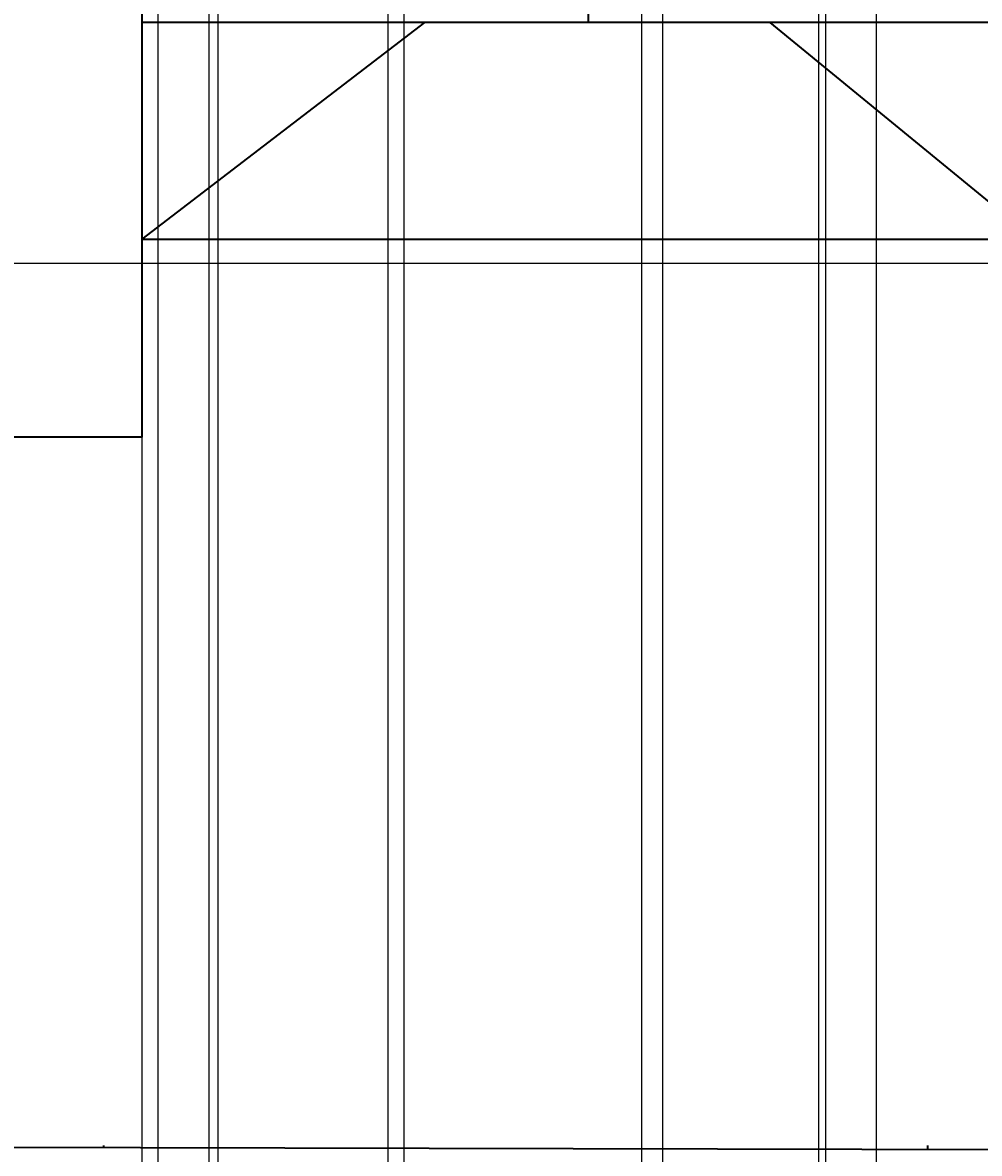
# Model space of a CAD drawing. Units: inches. Extents: x 27 to 200, y -50 to 102.
# Tile 17 of 26: x 117 to 145, y 19 to 52. Entities that reach past the tile are written whole.
import ezdxf

# ---------------------------------------------------------------- set-up
doc = ezdxf.new("R2010")
doc.units = ezdxf.units.IN
doc.header["$MEASUREMENT"] = 0
doc.layers.add('A-ANNO-DIMS', color=2, linetype='Continuous', lineweight=18)
doc.layers.add('A-ELEV', color=7, linetype='Continuous', lineweight=35)
doc.styles.get("Standard").update_dxf_attribs({"font": 'arial.ttf'})
doc.dimstyles.get("Standard").update_dxf_attribs({"dimtxt": 0.18, "dimasz": 0.18, "dimexe": 0.18, "dimexo": 0.0625, "dimgap": 0.09, "dimtad": 0, "dimtih": 1, "dimtoh": 1, "dimdec": 4, "dimzin": 0, "dimdsep": 46, "dimtxsty": 'Standard', "dimcen": 0.09, "dimadec": 0, "dimazin": 0, "dimtfac": 1, "dimtdec": 4, "dimtofl": 0, "dimtmove": 0, "dimatfit": 3, "dimfxl": 1, "dimtolj": 1, "dimtzin": 0, "dimarcsym": 0})

# ---------------------------------------------------------------- blocks, each defined once
blk = doc.blocks.new('*D48')
at = {"layer": 'A-ANNO-DIMS', "color": 0, "lineweight": -2, "transparency": 16777216}
for p, q in [((84.479, 44.926), (199.797, 44.926)), ((199.617, 44.746), (199.617, 14.26)), ((199.617, -16.589), (199.617, 13.897)), ((84.479, -16.769), (199.797, -16.769))]:
    blk.add_line(p, q, dxfattribs=at)
at = {"layer": 'A-ANNO-DIMS', "color": 0, "transparency": 16777216}
for points in [[(199.587, 44.746), (199.647, 44.746), (199.617, 44.926)], [(199.587, -16.589), (199.647, -16.589), (199.617, -16.769)]]:
    blk.add_solid(points, dxfattribs=at)
at = {"layer": 'Defpoints', "color": 0, "transparency": 16777216}
for p in [(84.417, 44.926), (199.617, 44.926), (84.417, -16.769)]:
    blk.add_point(p, dxfattribs=at)
at = {"layer": 'A-ANNO-DIMS', "color": 0, "transparency": 16777216, "insert": (199.617, 14.079), "char_height": 0.18, "attachment_point": 5}
blk.add_mtext('\\A1;61.7', dxfattribs=at)
blk = doc.blocks.new('*D51')
at = {"layer": 'A-ANNO-DIMS', "color": 0, "lineweight": -2, "transparency": 16777216}
for p, q in [((120.417, 45.561), (120.417, -25.149)), ((146.417, 45.561), (146.417, -25.149)), ((120.597, -24.969), (133.197, -24.969)), ((146.237, -24.969), (133.637, -24.969))]:
    blk.add_line(p, q, dxfattribs=at)
at = {"layer": 'A-ANNO-DIMS', "color": 0, "transparency": 16777216}
for points in [[(120.597, -24.939), (120.597, -24.999), (120.417, -24.969)], [(146.237, -24.939), (146.237, -24.999), (146.417, -24.969)]]:
    blk.add_solid(points, dxfattribs=at)
at = {"layer": 'Defpoints', "color": 0, "transparency": 16777216}
for p in [(120.417, 45.623), (146.417, 45.623), (146.417, -24.969)]:
    blk.add_point(p, dxfattribs=at)
at = {"layer": 'A-ANNO-DIMS', "color": 0, "transparency": 16777216, "insert": (133.417, -24.969), "char_height": 0.18, "attachment_point": 5}
blk.add_mtext('\\A1;26', dxfattribs=at)
blk = doc.blocks.new('*D53')
at = {"layer": 'A-ANNO-DIMS', "color": 0, "lineweight": -2, "transparency": 16777216}
for p, q in [((120.895, 14.04), (120.895, 102.306)), ((121.075, 102.126), (130.962, 102.126)), ((141.636, 102.126), (131.75, 102.126)), ((141.816, 14.04), (141.816, 102.306))]:
    blk.add_line(p, q, dxfattribs=at)
at = {"layer": 'A-ANNO-DIMS', "color": 0, "transparency": 16777216}
for points in [[(121.075, 102.156), (121.075, 102.096), (120.895, 102.126)], [(141.636, 102.156), (141.636, 102.096), (141.816, 102.126)]]:
    blk.add_solid(points, dxfattribs=at)
at = {"layer": 'Defpoints', "color": 0, "transparency": 16777216}
for p in [(141.816, 102.126), (120.895, 13.977), (141.816, 13.977)]:
    blk.add_point(p, dxfattribs=at)
at = {"layer": 'A-ANNO-DIMS', "color": 0, "transparency": 16777216, "insert": (131.356, 102.126), "char_height": 0.18, "attachment_point": 5}
blk.add_mtext('\\A1;20.92', dxfattribs=at)
blk = doc.blocks.new('*D57')
at = {"layer": 'A-ANNO-DIMS', "color": 0, "lineweight": -2, "transparency": 16777216}
for p, q in [((122.38, 4.48), (122.38, 102.306)), ((122.56, 102.126), (130.875, 102.126)), ((139.961, 102.126), (131.645, 102.126)), ((140.141, 4.48), (140.141, 102.306))]:
    blk.add_line(p, q, dxfattribs=at)
at = {"layer": 'A-ANNO-DIMS', "color": 0, "transparency": 16777216}
for points in [[(122.56, 102.156), (122.56, 102.096), (122.38, 102.126)], [(139.961, 102.156), (139.961, 102.096), (140.141, 102.126)]]:
    blk.add_solid(points, dxfattribs=at)
at = {"layer": 'Defpoints', "color": 0, "transparency": 16777216}
for p in [(140.141, 102.126), (122.38, 4.418), (140.141, 4.418)]:
    blk.add_point(p, dxfattribs=at)
at = {"layer": 'A-ANNO-DIMS', "color": 0, "transparency": 16777216, "insert": (131.26, 102.126), "char_height": 0.18, "attachment_point": 5}
blk.add_mtext('\\A1;17.76', dxfattribs=at)
blk = doc.blocks.new('*D59')
at = {"layer": 'A-ANNO-DIMS', "color": 0, "lineweight": -2, "transparency": 16777216}
for p, q in [((127.595, -0.162), (127.595, 102.306)), ((127.775, 102.126), (130.893, 102.126)), ((134.798, 102.126), (131.679, 102.126)), ((134.978, -0.162), (134.978, 102.306))]:
    blk.add_line(p, q, dxfattribs=at)
at = {"layer": 'A-ANNO-DIMS', "color": 0, "transparency": 16777216}
for points in [[(127.775, 102.156), (127.775, 102.096), (127.595, 102.126)], [(134.798, 102.156), (134.798, 102.096), (134.978, 102.126)]]:
    blk.add_solid(points, dxfattribs=at)
at = {"layer": 'Defpoints', "color": 0, "transparency": 16777216}
for p in [(134.978, 102.126), (127.595, -0.225), (134.978, -0.225)]:
    blk.add_point(p, dxfattribs=at)
at = {"layer": 'A-ANNO-DIMS', "color": 0, "transparency": 16777216, "insert": (131.286, 102.126), "char_height": 0.18, "attachment_point": 5}
blk.add_mtext('\\A1;7.383', dxfattribs=at)
blk = doc.blocks.new('*D61')
at = {"layer": 'A-ANNO-DIMS', "color": 0, "lineweight": -2, "transparency": 16777216}
for p, q in [((122.638, -4.237), (122.638, 102.306)), ((122.818, 102.126), (131.125, 102.126)), ((140.167, 102.126), (131.86, 102.126)), ((140.347, -4.237), (140.347, 102.306))]:
    blk.add_line(p, q, dxfattribs=at)
at = {"layer": 'A-ANNO-DIMS', "color": 0, "transparency": 16777216}
for points in [[(122.818, 102.156), (122.818, 102.096), (122.638, 102.126)], [(140.167, 102.156), (140.167, 102.096), (140.347, 102.126)]]:
    blk.add_solid(points, dxfattribs=at)
at = {"layer": 'Defpoints', "color": 0, "transparency": 16777216}
for p in [(140.347, 102.126), (122.638, -4.3), (140.347, -4.3)]:
    blk.add_point(p, dxfattribs=at)
at = {"layer": 'A-ANNO-DIMS', "color": 0, "transparency": 16777216, "insert": (131.493, 102.126), "char_height": 0.18, "attachment_point": 5}
blk.add_mtext('\\A1;17.71', dxfattribs=at)
blk = doc.blocks.new('*D63')
at = {"layer": 'A-ANNO-DIMS', "color": 0, "lineweight": -2, "transparency": 16777216}
for p, q in [((128.059, -9.034), (128.059, 102.306)), ((128.239, 102.126), (131.435, 102.126)), ((135.417, 102.126), (132.221, 102.126)), ((135.597, -9.034), (135.597, 102.306))]:
    blk.add_line(p, q, dxfattribs=at)
at = {"layer": 'A-ANNO-DIMS', "color": 0, "transparency": 16777216}
for points in [[(128.239, 102.156), (128.239, 102.096), (128.059, 102.126)], [(135.417, 102.156), (135.417, 102.096), (135.597, 102.126)]]:
    blk.add_solid(points, dxfattribs=at)
at = {"layer": 'Defpoints', "color": 0, "transparency": 16777216}
for p in [(135.597, 102.126), (128.059, -9.097), (135.597, -9.097)]:
    blk.add_point(p, dxfattribs=at)
at = {"layer": 'A-ANNO-DIMS', "color": 0, "transparency": 16777216, "insert": (131.828, 102.126), "char_height": 0.18, "attachment_point": 5}
blk.add_mtext('\\A1;7.538', dxfattribs=at)

msp = doc.modelspace()

# ---------------------------------------------------------------- linework, layer by layer
at = {"layer": 'A-ELEV'}
for p, q in [((120.4169, 87.9264), (120.4169, 51.9264)), ((133.4169, 87.9264), (133.4169, 51.9264)), ((146.4169, 51.9264), (120.4169, 51.9264)), ((128.6463, 51.9264), (120.4169, 45.6231)), ((146.4169, 45.6231), (138.7218, 51.9264)), ((120.4169, 45.6231), (146.4169, 45.6231)), ((191.4169, 19.002), (89.3118, 19.2307)), ((119.3118, 19.1635), (119.3118, 19.2307)), ((143.3118, 19.1097), (143.3118, 19.2307))]:
    msp.add_line(p, q, dxfattribs=at)
msp.add_lwpolyline([(84.4169, 65.5865), (120.4169, 65.5865), (120.4169, 39.8559), (84.4169, 39.8559)], close=True, dxfattribs=at)

# ---------------------------------------------------------------- dimensions: what is measured, and where the dimension line sits
at = {"layer": 'A-ANNO-DIMS'}
for base, p1, p2, override, picture, middle in [((141.8163, 102.1264), (120.8954, 13.9773), (141.8163, 13.9773), {"dimdec": 2, "dimlfac": 1, "dimrnd": 0, "dimzin": 0, "dimdsep": 46, "dimlunit": 2}, '*D53', (131.3558, 102.1264)), ((140.1406, 102.1264), (122.38, 4.4177), (140.1406, 4.4177), {"dimdec": 2, "dimlfac": 1, "dimrnd": 0, "dimzin": 0, "dimdsep": 46, "dimlunit": 2}, '*D57', (131.2603, 102.1264)), ((140.3471, 102.1264), (122.6381, -4.2997), (140.3471, -4.2997), {"dimdec": 2, "dimlfac": 1, "dimrnd": 0, "dimzin": 0, "dimdsep": 46, "dimlunit": 2}, '*D61', (131.4926, 102.1264)), ((134.9776, 102.1264), (127.5946, -0.2247), (134.9776, -0.2247), {"dimdec": 3, "dimlfac": 1, "dimrnd": 0, "dimzin": 0, "dimdsep": 46, "dimlunit": 2}, '*D59', (131.2861, 102.1264)), ((135.5972, 102.1264), (128.0592, -9.0968), (135.5972, -9.0968), {"dimdec": 3, "dimlfac": 1, "dimrnd": 0, "dimzin": 0, "dimdsep": 46, "dimlunit": 2}, '*D63', (131.8282, 102.1264)), ((146.4169, -24.9693), (120.4169, 45.6231), (146.4169, 45.6231), {"dimdec": 0, "dimlfac": 1, "dimrnd": 0, "dimzin": 0, "dimdsep": 46, "dimlunit": 2}, '*D51', (133.4169, -24.9693))]:
    dim = msp.add_linear_dim(base=base, p1=p1, p2=p2, dimstyle='Standard', override=override, dxfattribs=at)
    dim.commit()
    dim.dimension.update_dxf_attribs({"geometry": picture, "text_midpoint": middle})
dim = msp.add_linear_dim(base=(199.6169, 44.9264), p1=(84.4169, -16.7693), p2=(84.4169, 44.9264), angle=90, dimstyle='Standard', override={"dimdec": 1, "dimlfac": 1, "dimrnd": 0, "dimzin": 0, "dimdsep": 46, "dimlunit": 2}, dxfattribs=at)
dim.commit()
dim.dimension.update_dxf_attribs({"geometry": '*D48', "text_midpoint": (199.6169, 14.0786)})

doc.saveas('drawing.dxf')
